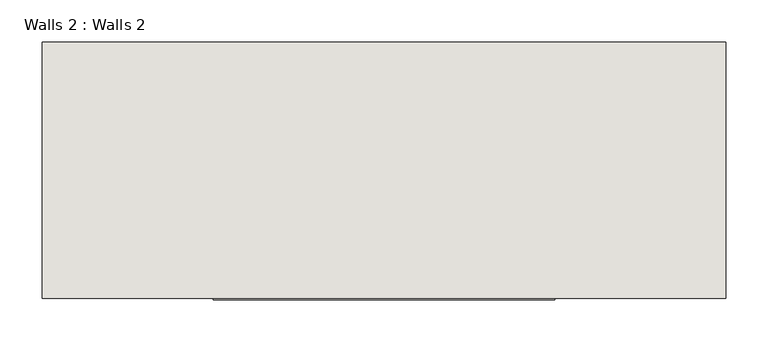
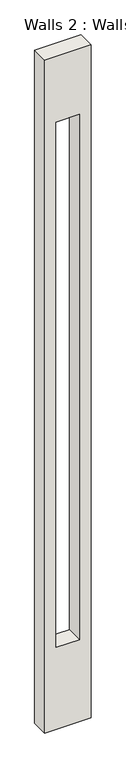
"""IFC4 building model written with IfcOpenShell, lengths in millimetres: wall geometry, Walls 2 : Walls 2."""

from ifc_helpers import new_model, si_unit, frame, origin, place, context, project, spatial, polyline, outline, extrude, source, transform, mapped, element, save


def walls_2_walls_2_726db825(model_context):
    return source(origin(), model_context, "Body", "SweptSolid", [
        extrude(outline(polyline([(15240.0, -2168.7569651), (15240.0, -2981.5569651), (2743.2, -2981.5569651), (2743.2, -2168.7569651), (15240.0, -2168.7569651)]), holes=[polyline([(14020.8, -2778.3569651), (14020.8, -2371.9569651), (4267.2, -2371.9569651), (4267.2, -2778.3569651), (14020.8, -2778.3569651)])]), frame((0.0, 146.7055142, 0.0), z_axis=(0.0, 1.0, 0.0), x_axis=(0.0, 0.0, 1.0)), (0.0, 0.0, 1.0), 304.8),
    ])


if __name__ == "__main__":
    model = new_model("IFC4")
    model_context = context("Model", 3, world=origin())
    ifc_project = project(units=[si_unit("LENGTHUNIT", "METRE", prefix="MILLI")], contexts=[model_context])
    site = spatial("IfcSite", under=ifc_project)
    building = spatial("IfcBuilding", under=site)
    placement = place(None, origin())
    walls_2_walls_2_shape = walls_2_walls_2_726db825(model_context)
    element("IfcWall", 1, ObjectType="Walls 2 : Walls 2", at=placement, inside=building, context=model_context, shape_type="MappedRepresentation", body=[
        mapped(walls_2_walls_2_shape, transform((0.0, 0.0, 0.0), x_axis=(1.0, 0.0, 0.0), y_axis=(0.0, 1.0, 0.0), z_axis=(0.0, 0.0, 1.0))),
    ])
    save(model, "model.ifc")

# Revit data of these elements
# Element 1 (IfcWall, "Walls 2 : Walls 2")
#   Materials on its faces: "1 wall white", "Default Wall"
# Materials
#   "1 wall white": class "Generic", colour RGB 244 245 241, transparency 0, Cost = 0
#   "Default Wall": colour RGB 128 128 128, transparency 0, Cost = 0
